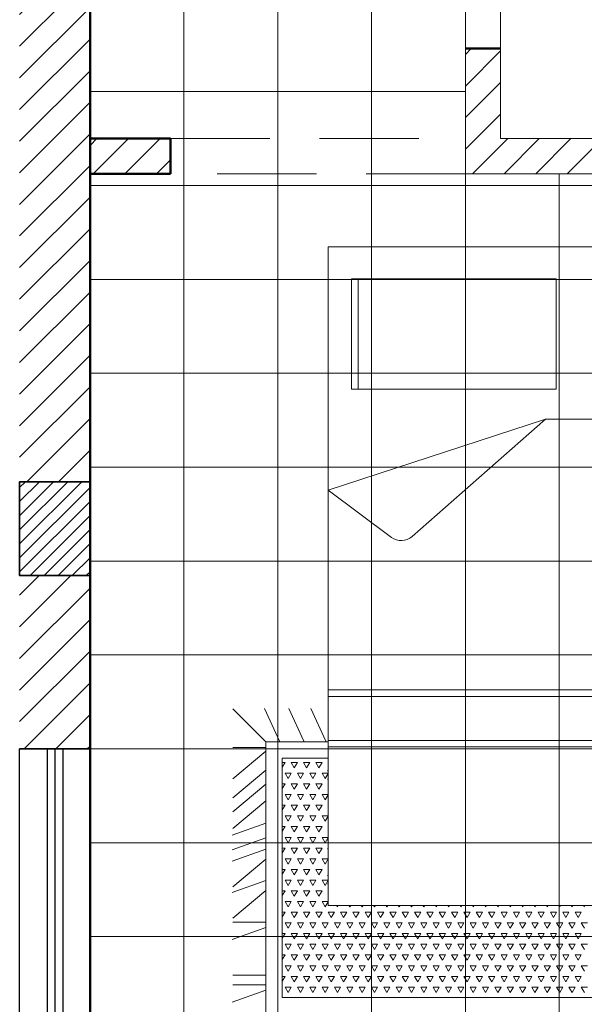
# Model space of a CAD drawing. Units: millimetres. Extents: x 225995 to 227247, y 225507 to 226008.
# Tile 14 of 23: x 226749 to 226821, y 225755 to 225881. Entities that reach past the tile are written whole.
import ezdxf

# ---------------------------------------------------------------- set-up
doc = ezdxf.new("R2010")
doc.units = ezdxf.units.MM
doc.linetypes.add('DASHED', pattern=[19.05, 12.7, -6.35])
for name, color, linetype, lineweight in [('A-COLS', 40, 'Continuous', 35), ('A-FLOR-PATT', 8, 'Continuous', 13), ('A-FURN', 9, 'Continuous', 18), ('A-GLAZ', 4, 'Continuous', 25), ('A-WALL', 7, 'Continuous', 50), ('A-WALL-OVHD', 1, 'DASHED', 18), ('A-WALL-PATT', 8, 'Continuous', 13)]:
    doc.layers.add(name, color=color, linetype=linetype, lineweight=lineweight)

# ---------------------------------------------------------------- blocks, each defined once
blk = doc.blocks.new('A$C6D2A2628')
for p, q in [((0.291, 2.4297), (1.791, 2.4297)), ((0.291, 0.4297), (0.291, 2.4297)), ((0.3622, 2.3321), (0.9834, 2.3321)), ((0.3622, 1.9967), (0.3622, 2.3321)), ((0.3822, 1.9967), (0.3822, 2.3321)), ((0.9834, 2.3321), (0.9834, 1.9967)), ((0.9834, 1.9967), (0.3622, 1.9967)), ((0.291, 1.6908), (0.9515, 1.9058)), ((0.9515, 1.9058), (0.5462, 1.5497)), ((0.9515, 1.9058), (1.1116, 1.9058)), ((0.4832, 1.5472), (0.291, 1.6908)), ((0.291, 1.0837), (1.791, 1.0837)), ((0.291, 1.0637), (1.791, 1.0637)), ((0.1019, 0.9267), (0.0019, 1.0267)), ((0.0977, 1.0278), (0.1431, 0.9278)), ((0.1716, 1.0278), (0.217, 0.9278)), ((0.2388, 1.0278), (0.2843, 0.9278)), ((0.291, 0.9307), (1.791, 0.9307)), ((0.0015, 0.9091), (0.1015, 0.9091)), ((0.0015, 0.8141), (0.1015, 0.8978)), ((0.291, 0.9267), (0.1019, 0.9267)), ((0.1019, 0.9267), (0.1019, 0.1)), ((0.291, 0.9107), (1.791, 0.9107)), ((0.291, 0.8767), (0.1519, 0.8767)), ((0.1519, 0.8767), (0.1519, 0.15)), ((0.0015, 0.7564), (0.1015, 0.84)), ((0.1519, 0.8494), (0.1601, 0.8636)), ((0.1519, 0.8636), (0.1601, 0.8636)), ((0.1882, 0.8473), (0.1788, 0.8636)), ((0.1788, 0.8636), (0.1976, 0.8636)), ((0.1882, 0.8473), (0.1976, 0.8636)), ((0.2257, 0.8473), (0.2163, 0.8636)), ((0.2163, 0.8636), (0.2351, 0.8636)), ((0.2257, 0.8473), (0.2351, 0.8636)), ((0.2632, 0.8473), (0.2538, 0.8636)), ((0.2538, 0.8636), (0.2726, 0.8636)), ((0.2632, 0.8473), (0.2726, 0.8636)), ((0.291, 0.8376), (0.2893, 0.8393)), ((0.1695, 0.8148), (0.1601, 0.8311)), ((0.1601, 0.8311), (0.1788, 0.8311)), ((0.1695, 0.8148), (0.1788, 0.8311)), ((0.207, 0.8148), (0.1976, 0.8311)), ((0.1976, 0.8311), (0.2163, 0.8311)), ((0.207, 0.8148), (0.2163, 0.8311)), ((0.2445, 0.8148), (0.2351, 0.8311)), ((0.2351, 0.8311), (0.2538, 0.8311)), ((0.2445, 0.8148), (0.2538, 0.8311)), ((0.282, 0.8148), (0.2726, 0.8311)), ((0.2726, 0.8311), (0.291, 0.8311)), ((0.282, 0.8148), (0.291, 0.8305)), ((0.291, 0.8144), (0.2893, 0.8128)), ((0.0015, 0.7139), (0.1015, 0.7975)), ((0.1519, 0.7844), (0.1601, 0.7986)), ((0.1519, 0.7986), (0.1601, 0.7986)), ((0.1882, 0.7824), (0.1788, 0.7986)), ((0.1788, 0.7986), (0.1976, 0.7986)), ((0.1882, 0.7824), (0.1976, 0.7986)), ((0.2257, 0.7824), (0.2163, 0.7986)), ((0.2163, 0.7986), (0.2351, 0.7986)), ((0.2257, 0.7824), (0.2351, 0.7986)), ((0.2632, 0.7824), (0.2538, 0.7986)), ((0.2538, 0.7986), (0.2726, 0.7986)), ((0.2632, 0.7824), (0.2726, 0.7986)), ((0.1695, 0.7499), (0.1601, 0.7661)), ((0.1601, 0.7661), (0.1788, 0.7661)), ((0.1695, 0.7499), (0.1788, 0.7661)), ((0.207, 0.7499), (0.1976, 0.7661)), ((0.1976, 0.7661), (0.2163, 0.7661)), ((0.207, 0.7499), (0.2163, 0.7661)), ((0.2445, 0.7499), (0.2351, 0.7661)), ((0.2351, 0.7661), (0.2538, 0.7661)), ((0.2445, 0.7499), (0.2538, 0.7661)), ((0.282, 0.7499), (0.2726, 0.7661)), ((0.2726, 0.7661), (0.291, 0.7661)), ((0.282, 0.7499), (0.291, 0.7655)), ((0.0015, 0.6633), (0.1015, 0.7469)), ((0.1519, 0.7195), (0.1601, 0.7337)), ((0.1519, 0.7337), (0.1601, 0.7337)), ((0.1882, 0.7174), (0.1788, 0.7337)), ((0.1788, 0.7337), (0.1976, 0.7337)), ((0.1882, 0.7174), (0.1976, 0.7337)), ((0.2257, 0.7174), (0.2163, 0.7337)), ((0.2163, 0.7337), (0.2351, 0.7337)), ((0.2257, 0.7174), (0.2351, 0.7337)), ((0.2632, 0.7174), (0.2538, 0.7337)), ((0.2538, 0.7337), (0.2726, 0.7337)), ((0.2632, 0.7174), (0.2726, 0.7337)), ((0.1695, 0.6849), (0.1601, 0.7012)), ((0.1601, 0.7012), (0.1788, 0.7012)), ((0.1695, 0.6849), (0.1788, 0.7012)), ((0.207, 0.6849), (0.1976, 0.7012)), ((0.1976, 0.7012), (0.2163, 0.7012)), ((0.207, 0.6849), (0.2163, 0.7012)), ((0.2445, 0.6849), (0.2351, 0.7012)), ((0.2351, 0.7012), (0.2538, 0.7012)), ((0.2445, 0.6849), (0.2538, 0.7012)), ((0.282, 0.6849), (0.2726, 0.7012)), ((0.2726, 0.7012), (0.291, 0.7012)), ((0.282, 0.6849), (0.291, 0.7006)), ((0, 0.6428), (0.1015, 0.6794)), ((0.1519, 0.6545), (0.1601, 0.6687)), ((0.1519, 0.6687), (0.1601, 0.6687)), ((0.1882, 0.6525), (0.1788, 0.6687)), ((0.1788, 0.6687), (0.1976, 0.6687)), ((0.1882, 0.6525), (0.1976, 0.6687)), ((0.2257, 0.6525), (0.2163, 0.6687)), ((0.2163, 0.6687), (0.2351, 0.6687)), ((0.2257, 0.6525), (0.2351, 0.6687)), ((0.2632, 0.6525), (0.2538, 0.6687)), ((0.2538, 0.6687), (0.2726, 0.6687)), ((0.2632, 0.6525), (0.2726, 0.6687)), ((0, 0.5984), (0.1015, 0.6351)), ((0.1695, 0.62), (0.1601, 0.6362)), ((0.1601, 0.6362), (0.1788, 0.6362)), ((0.1695, 0.62), (0.1788, 0.6362)), ((0.207, 0.62), (0.1976, 0.6362)), ((0.1976, 0.6362), (0.2163, 0.6362)), ((0.207, 0.62), (0.2163, 0.6362)), ((0.2445, 0.62), (0.2351, 0.6362)), ((0.2351, 0.6362), (0.2538, 0.6362)), ((0.2445, 0.62), (0.2538, 0.6362)), ((0.282, 0.62), (0.2726, 0.6362)), ((0.2726, 0.6362), (0.291, 0.6362)), ((0.282, 0.62), (0.291, 0.6356)), ((0, 0.5636), (0.1015, 0.6003)), ((0.1519, 0.5896), (0.1601, 0.6037)), ((0.1519, 0.6037), (0.1601, 0.6037)), ((0.1882, 0.5875), (0.1788, 0.6037)), ((0.1788, 0.6037), (0.1976, 0.6037)), ((0.1882, 0.5875), (0.1976, 0.6037)), ((0.2257, 0.5875), (0.2163, 0.6037)), ((0.2163, 0.6037), (0.2351, 0.6037)), ((0.2257, 0.5875), (0.2351, 0.6037)), ((0.2632, 0.5875), (0.2538, 0.6037)), ((0.2538, 0.6037), (0.2726, 0.6037)), ((0.2632, 0.5875), (0.2726, 0.6037)), ((0.291, 0.6255), (0.2893, 0.6271)), ((0.291, 0.6023), (0.2893, 0.6006)), ((0.0015, 0.4859), (0.1015, 0.5695)), ((0.1695, 0.555), (0.1601, 0.5713)), ((0.1601, 0.5713), (0.1788, 0.5713)), ((0.1695, 0.555), (0.1788, 0.5713)), ((0.207, 0.555), (0.1976, 0.5713)), ((0.1976, 0.5713), (0.2163, 0.5713)), ((0.207, 0.555), (0.2163, 0.5713)), ((0.2445, 0.555), (0.2351, 0.5713)), ((0.2351, 0.5713), (0.2538, 0.5713)), ((0.2445, 0.555), (0.2538, 0.5713)), ((0.282, 0.555), (0.2726, 0.5713)), ((0.2726, 0.5713), (0.291, 0.5713)), ((0.282, 0.555), (0.291, 0.5707)), ((0.1519, 0.5246), (0.1601, 0.5388)), ((0.1519, 0.5388), (0.1601, 0.5388)), ((0.1882, 0.5226), (0.1788, 0.5388)), ((0.1788, 0.5388), (0.1976, 0.5388)), ((0.1882, 0.5226), (0.1976, 0.5388)), ((0.2257, 0.5226), (0.2163, 0.5388)), ((0.2163, 0.5388), (0.2351, 0.5388)), ((0.2257, 0.5226), (0.2351, 0.5388)), ((0.2632, 0.5226), (0.2538, 0.5388)), ((0.2538, 0.5388), (0.2726, 0.5388)), ((0.2632, 0.5226), (0.2726, 0.5388)), ((0.291, 0.5194), (0.2893, 0.5211)), ((0, 0.4686), (0.1015, 0.5053)), ((0.1695, 0.4901), (0.1601, 0.5063)), ((0.1601, 0.5063), (0.1788, 0.5063)), ((0.1695, 0.4901), (0.1788, 0.5063)), ((0.207, 0.4901), (0.1976, 0.5063)), ((0.1976, 0.5063), (0.2163, 0.5063)), ((0.207, 0.4901), (0.2163, 0.5063)), ((0.2445, 0.4901), (0.2351, 0.5063)), ((0.2351, 0.5063), (0.2538, 0.5063)), ((0.2445, 0.4901), (0.2538, 0.5063)), ((0.282, 0.4901), (0.2726, 0.5063)), ((0.2726, 0.5063), (0.291, 0.5063)), ((0.282, 0.4901), (0.291, 0.5057)), ((0.291, 0.4962), (0.2893, 0.4946)), ((0.0015, 0.3909), (0.1015, 0.4745)), ((0.1519, 0.4597), (0.1601, 0.4738)), ((0.1519, 0.4738), (0.1601, 0.4738)), ((0.1882, 0.4576), (0.1788, 0.4738)), ((0.1788, 0.4738), (0.1976, 0.4738)), ((0.1882, 0.4576), (0.1976, 0.4738)), ((0.2257, 0.4576), (0.2163, 0.4738)), ((0.2163, 0.4738), (0.2351, 0.4738)), ((0.2257, 0.4576), (0.2351, 0.4738)), ((0.2632, 0.4576), (0.2538, 0.4738)), ((0.2538, 0.4738), (0.2726, 0.4738)), ((0.2632, 0.4576), (0.2726, 0.4738)), ((0.1695, 0.4251), (0.1601, 0.4414)), ((0.1601, 0.4414), (0.1788, 0.4414)), ((0.1695, 0.4251), (0.1788, 0.4414)), ((0.207, 0.4251), (0.1976, 0.4414)), ((0.1976, 0.4414), (0.2163, 0.4414)), ((0.207, 0.4251), (0.2163, 0.4414)), ((0.2445, 0.4251), (0.2351, 0.4414)), ((0.2351, 0.4414), (0.2538, 0.4414)), ((0.2445, 0.4251), (0.2538, 0.4414)), ((0.282, 0.4251), (0.2726, 0.4414)), ((0.2726, 0.4414), (0.291, 0.4414)), ((0.282, 0.4251), (0.291, 0.4408)), ((1.791, 0.4297), (0.291, 0.4297)), ((0.3195, 0.4251), (0.3168, 0.4297)), ((0.3195, 0.4251), (0.3221, 0.4297)), ((0.357, 0.4251), (0.3543, 0.4297)), ((0.357, 0.4251), (0.3596, 0.4297)), ((0.3945, 0.4251), (0.3918, 0.4297)), ((0.3945, 0.4251), (0.3971, 0.4297)), ((0.432, 0.4251), (0.4293, 0.4297)), ((0.432, 0.4251), (0.4346, 0.4297)), ((0.4695, 0.4251), (0.4668, 0.4297)), ((0.4695, 0.4251), (0.4721, 0.4297)), ((0.507, 0.4251), (0.5043, 0.4297)), ((0.507, 0.4251), (0.5096, 0.4297)), ((0.5445, 0.4251), (0.5418, 0.4297)), ((0.5445, 0.4251), (0.5471, 0.4297)), ((0.582, 0.4251), (0.5793, 0.4297)), ((0.582, 0.4251), (0.5846, 0.4297)), ((0.6195, 0.4251), (0.6168, 0.4297)), ((0.6195, 0.4251), (0.6221, 0.4297)), ((0.657, 0.4251), (0.6543, 0.4297)), ((0.657, 0.4251), (0.6596, 0.4297)), ((0.6945, 0.4251), (0.6918, 0.4297)), ((0.6945, 0.4251), (0.6971, 0.4297)), ((0.732, 0.4251), (0.7293, 0.4297)), ((0.732, 0.4251), (0.7346, 0.4297)), ((0.7695, 0.4251), (0.7668, 0.4297)), ((0.7695, 0.4251), (0.7721, 0.4297)), ((0.807, 0.4251), (0.8043, 0.4297)), ((0.807, 0.4251), (0.8096, 0.4297)), ((0.8445, 0.4251), (0.8418, 0.4297)), ((0.8445, 0.4251), (0.8471, 0.4297)), ((0.882, 0.4251), (0.8793, 0.4297)), ((0.882, 0.4251), (0.8846, 0.4297)), ((0.9195, 0.4251), (0.9168, 0.4297)), ((0.9195, 0.4251), (0.9221, 0.4297)), ((0.957, 0.4251), (0.9543, 0.4297)), ((0.957, 0.4251), (0.9596, 0.4297)), ((0.9945, 0.4251), (0.9918, 0.4297)), ((0.9945, 0.4251), (0.9971, 0.4297)), ((1.032, 0.4251), (1.0293, 0.4297)), ((1.032, 0.4251), (1.0346, 0.4297)), ((1.0695, 0.4251), (1.0668, 0.4297)), ((0.1519, 0.3947), (0.1601, 0.4089)), ((0.1519, 0.4089), (0.1601, 0.4089)), ((0.1882, 0.3927), (0.1788, 0.4089)), ((0.1788, 0.4089), (0.1976, 0.4089)), ((0.1882, 0.3927), (0.1976, 0.4089)), ((0.2257, 0.3927), (0.2163, 0.4089)), ((0.2163, 0.4089), (0.2351, 0.4089)), ((0.2257, 0.3927), (0.2351, 0.4089)), ((0.2632, 0.3927), (0.2538, 0.4089)), ((0.2538, 0.4089), (0.2726, 0.4089)), ((0.2632, 0.3927), (0.2726, 0.4089)), ((0.3007, 0.3927), (0.2913, 0.4089)), ((0.2913, 0.4089), (0.3101, 0.4089)), ((0.3007, 0.3927), (0.3101, 0.4089)), ((0.3382, 0.3927), (0.3288, 0.4089)), ((0.3288, 0.4089), (0.3476, 0.4089)), ((0.3382, 0.3927), (0.3476, 0.4089)), ((0.3757, 0.3927), (0.3663, 0.4089)), ((0.3663, 0.4089), (0.3851, 0.4089)), ((0.3757, 0.3927), (0.3851, 0.4089)), ((0.4132, 0.3927), (0.4038, 0.4089)), ((0.4038, 0.4089), (0.4226, 0.4089)), ((0.4132, 0.3927), (0.4226, 0.4089)), ((0.4507, 0.3927), (0.4413, 0.4089)), ((0.4413, 0.4089), (0.4601, 0.4089)), ((0.4507, 0.3927), (0.4601, 0.4089)), ((0.4882, 0.3927), (0.4788, 0.4089)), ((0.4788, 0.4089), (0.4976, 0.4089)), ((0.4882, 0.3927), (0.4976, 0.4089)), ((0.5257, 0.3927), (0.5163, 0.4089)), ((0.5163, 0.4089), (0.5351, 0.4089)), ((0.5257, 0.3927), (0.5351, 0.4089)), ((0.5632, 0.3927), (0.5538, 0.4089)), ((0.5538, 0.4089), (0.5726, 0.4089)), ((0.5632, 0.3927), (0.5726, 0.4089)), ((0.6007, 0.3927), (0.5913, 0.4089)), ((0.5913, 0.4089), (0.6101, 0.4089)), ((0.6007, 0.3927), (0.6101, 0.4089)), ((0.6382, 0.3927), (0.6288, 0.4089)), ((0.6288, 0.4089), (0.6476, 0.4089)), ((0.6382, 0.3927), (0.6476, 0.4089)), ((0.6757, 0.3927), (0.6663, 0.4089)), ((0.6663, 0.4089), (0.6851, 0.4089)), ((0.6757, 0.3927), (0.6851, 0.4089)), ((0.7132, 0.3927), (0.7038, 0.4089)), ((0.7038, 0.4089), (0.7226, 0.4089)), ((0.7132, 0.3927), (0.7226, 0.4089)), ((0.7507, 0.3927), (0.7413, 0.4089)), ((0.7413, 0.4089), (0.7601, 0.4089)), ((0.7507, 0.3927), (0.7601, 0.4089)), ((0.7882, 0.3927), (0.7788, 0.4089)), ((0.7788, 0.4089), (0.7976, 0.4089)), ((0.7882, 0.3927), (0.7976, 0.4089)), ((0.8257, 0.3927), (0.8163, 0.4089)), ((0.8163, 0.4089), (0.8351, 0.4089)), ((0.8257, 0.3927), (0.8351, 0.4089)), ((0.8632, 0.3927), (0.8538, 0.4089)), ((0.8538, 0.4089), (0.8726, 0.4089)), ((0.8632, 0.3927), (0.8726, 0.4089)), ((0.9007, 0.3927), (0.8913, 0.4089)), ((0.8913, 0.4089), (0.9101, 0.4089)), ((0.9007, 0.3927), (0.9101, 0.4089)), ((0.9382, 0.3927), (0.9288, 0.4089)), ((0.9288, 0.4089), (0.9476, 0.4089)), ((0.9382, 0.3927), (0.9476, 0.4089)), ((0.9757, 0.3927), (0.9663, 0.4089)), ((0.9663, 0.4089), (0.9851, 0.4089)), ((0.9757, 0.3927), (0.9851, 0.4089)), ((1.0132, 0.3927), (1.0038, 0.4089)), ((1.0038, 0.4089), (1.0226, 0.4089)), ((1.0132, 0.3927), (1.0226, 0.4089)), ((1.0507, 0.3927), (1.0413, 0.4089)), ((1.0413, 0.4089), (1.0601, 0.4089)), ((1.0507, 0.3927), (1.0601, 0.4089)), ((0, 0.3261), (0.1015, 0.3628)), ((0.0015, 0.3783), (0.1015, 0.3783)), ((0.1695, 0.3602), (0.1601, 0.3764)), ((0.1601, 0.3764), (0.1788, 0.3764)), ((0.1695, 0.3602), (0.1788, 0.3764)), ((0.207, 0.3602), (0.1976, 0.3764)), ((0.1976, 0.3764), (0.2163, 0.3764)), ((0.207, 0.3602), (0.2163, 0.3764)), ((0.2445, 0.3602), (0.2351, 0.3764)), ((0.2351, 0.3764), (0.2538, 0.3764)), ((0.2445, 0.3602), (0.2538, 0.3764)), ((0.282, 0.3602), (0.2726, 0.3764)), ((0.2726, 0.3764), (0.2913, 0.3764)), ((0.282, 0.3602), (0.2913, 0.3764)), ((0.3195, 0.3602), (0.3101, 0.3764)), ((0.3101, 0.3764), (0.3288, 0.3764)), ((0.3195, 0.3602), (0.3288, 0.3764)), ((0.357, 0.3602), (0.3476, 0.3764)), ((0.3476, 0.3764), (0.3663, 0.3764)), ((0.357, 0.3602), (0.3663, 0.3764)), ((0.3945, 0.3602), (0.3851, 0.3764)), ((0.3851, 0.3764), (0.4038, 0.3764)), ((0.3945, 0.3602), (0.4038, 0.3764)), ((0.432, 0.3602), (0.4226, 0.3764)), ((0.4226, 0.3764), (0.4413, 0.3764)), ((0.432, 0.3602), (0.4413, 0.3764)), ((0.4695, 0.3602), (0.4601, 0.3764)), ((0.4601, 0.3764), (0.4788, 0.3764)), ((0.4695, 0.3602), (0.4788, 0.3764)), ((0.507, 0.3602), (0.4976, 0.3764)), ((0.4976, 0.3764), (0.5163, 0.3764)), ((0.507, 0.3602), (0.5163, 0.3764)), ((0.5445, 0.3602), (0.5351, 0.3764)), ((0.5351, 0.3764), (0.5538, 0.3764)), ((0.5445, 0.3602), (0.5538, 0.3764)), ((0.582, 0.3602), (0.5726, 0.3764)), ((0.5726, 0.3764), (0.5913, 0.3764)), ((0.582, 0.3602), (0.5913, 0.3764)), ((0.6195, 0.3602), (0.6101, 0.3764)), ((0.6101, 0.3764), (0.6288, 0.3764)), ((0.6195, 0.3602), (0.6288, 0.3764)), ((0.657, 0.3602), (0.6476, 0.3764)), ((0.6476, 0.3764), (0.6663, 0.3764)), ((0.657, 0.3602), (0.6663, 0.3764)), ((0.6945, 0.3602), (0.6851, 0.3764)), ((0.6851, 0.3764), (0.7038, 0.3764)), ((0.6945, 0.3602), (0.7038, 0.3764)), ((0.732, 0.3602), (0.7226, 0.3764)), ((0.7226, 0.3764), (0.7413, 0.3764)), ((0.732, 0.3602), (0.7413, 0.3764)), ((0.7695, 0.3602), (0.7601, 0.3764)), ((0.7601, 0.3764), (0.7788, 0.3764)), ((0.7695, 0.3602), (0.7788, 0.3764)), ((0.807, 0.3602), (0.7976, 0.3764)), ((0.7976, 0.3764), (0.8163, 0.3764)), ((0.807, 0.3602), (0.8163, 0.3764)), ((0.8445, 0.3602), (0.8351, 0.3764)), ((0.8351, 0.3764), (0.8538, 0.3764)), ((0.8445, 0.3602), (0.8538, 0.3764)), ((0.882, 0.3602), (0.8726, 0.3764)), ((0.8726, 0.3764), (0.8913, 0.3764)), ((0.882, 0.3602), (0.8913, 0.3764)), ((0.9195, 0.3602), (0.9101, 0.3764)), ((0.9101, 0.3764), (0.9288, 0.3764)), ((0.9195, 0.3602), (0.9288, 0.3764)), ((0.957, 0.3602), (0.9476, 0.3764)), ((0.9476, 0.3764), (0.9663, 0.3764)), ((0.957, 0.3602), (0.9663, 0.3764)), ((0.9945, 0.3602), (0.9851, 0.3764)), ((0.9851, 0.3764), (1.0038, 0.3764)), ((0.9945, 0.3602), (1.0038, 0.3764)), ((1.032, 0.3602), (1.0226, 0.3764)), ((1.0226, 0.3764), (1.0413, 0.3764)), ((1.032, 0.3602), (1.0413, 0.3764)), ((1.0695, 0.3602), (1.0601, 0.3764)), ((1.0601, 0.3764), (1.0788, 0.3764)), ((0.1519, 0.3298), (0.1601, 0.3439)), ((0.1519, 0.3439), (0.1601, 0.3439)), ((0.1882, 0.3277), (0.1788, 0.3439)), ((0.1788, 0.3439), (0.1976, 0.3439)), ((0.1882, 0.3277), (0.1976, 0.3439)), ((0.2257, 0.3277), (0.2163, 0.3439)), ((0.2163, 0.3439), (0.2351, 0.3439)), ((0.2257, 0.3277), (0.2351, 0.3439)), ((0.2632, 0.3277), (0.2538, 0.3439)), ((0.2538, 0.3439), (0.2726, 0.3439)), ((0.2632, 0.3277), (0.2726, 0.3439)), ((0.3007, 0.3277), (0.2913, 0.3439)), ((0.2913, 0.3439), (0.3101, 0.3439)), ((0.3007, 0.3277), (0.3101, 0.3439)), ((0.3382, 0.3277), (0.3288, 0.3439)), ((0.3288, 0.3439), (0.3476, 0.3439)), ((0.3382, 0.3277), (0.3476, 0.3439)), ((0.3757, 0.3277), (0.3663, 0.3439)), ((0.3663, 0.3439), (0.3851, 0.3439)), ((0.3757, 0.3277), (0.3851, 0.3439)), ((0.4132, 0.3277), (0.4038, 0.3439)), ((0.4038, 0.3439), (0.4226, 0.3439)), ((0.4132, 0.3277), (0.4226, 0.3439)), ((0.4507, 0.3277), (0.4413, 0.3439)), ((0.4413, 0.3439), (0.4601, 0.3439)), ((0.4507, 0.3277), (0.4601, 0.3439)), ((0.4882, 0.3277), (0.4788, 0.3439)), ((0.4788, 0.3439), (0.4976, 0.3439)), ((0.4882, 0.3277), (0.4976, 0.3439)), ((0.5257, 0.3277), (0.5163, 0.3439)), ((0.5163, 0.3439), (0.5351, 0.3439)), ((0.5257, 0.3277), (0.5351, 0.3439)), ((0.5632, 0.3277), (0.5538, 0.3439)), ((0.5538, 0.3439), (0.5726, 0.3439)), ((0.5632, 0.3277), (0.5726, 0.3439)), ((0.6007, 0.3277), (0.5913, 0.3439)), ((0.5913, 0.3439), (0.6101, 0.3439)), ((0.6007, 0.3277), (0.6101, 0.3439)), ((0.6382, 0.3277), (0.6288, 0.3439)), ((0.6288, 0.3439), (0.6476, 0.3439)), ((0.6382, 0.3277), (0.6476, 0.3439)), ((0.6757, 0.3277), (0.6663, 0.3439)), ((0.6663, 0.3439), (0.6851, 0.3439)), ((0.6757, 0.3277), (0.6851, 0.3439)), ((0.7132, 0.3277), (0.7038, 0.3439)), ((0.7038, 0.3439), (0.7226, 0.3439)), ((0.7132, 0.3277), (0.7226, 0.3439)), ((0.7507, 0.3277), (0.7413, 0.3439)), ((0.7413, 0.3439), (0.7601, 0.3439)), ((0.7507, 0.3277), (0.7601, 0.3439)), ((0.7882, 0.3277), (0.7788, 0.3439)), ((0.7788, 0.3439), (0.7976, 0.3439)), ((0.7882, 0.3277), (0.7976, 0.3439)), ((0.8257, 0.3277), (0.8163, 0.3439)), ((0.8163, 0.3439), (0.8351, 0.3439)), ((0.8257, 0.3277), (0.8351, 0.3439)), ((0.8632, 0.3277), (0.8538, 0.3439)), ((0.8538, 0.3439), (0.8726, 0.3439)), ((0.8632, 0.3277), (0.8726, 0.3439)), ((0.9007, 0.3277), (0.8913, 0.3439)), ((0.8913, 0.3439), (0.9101, 0.3439)), ((0.9007, 0.3277), (0.9101, 0.3439)), ((0.9382, 0.3277), (0.9288, 0.3439)), ((0.9288, 0.3439), (0.9476, 0.3439)), ((0.9382, 0.3277), (0.9476, 0.3439)), ((0.9757, 0.3277), (0.9663, 0.3439)), ((0.9663, 0.3439), (0.9851, 0.3439)), ((0.9757, 0.3277), (0.9851, 0.3439)), ((1.0132, 0.3277), (1.0038, 0.3439)), ((1.0038, 0.3439), (1.0226, 0.3439)), ((1.0132, 0.3277), (1.0226, 0.3439)), ((1.0507, 0.3277), (1.0413, 0.3439)), ((1.0413, 0.3439), (1.0601, 0.3439)), ((1.0507, 0.3277), (1.0601, 0.3439)), ((0.1695, 0.2952), (0.1601, 0.3115)), ((0.1601, 0.3115), (0.1788, 0.3115)), ((0.1695, 0.2952), (0.1788, 0.3115)), ((0.207, 0.2952), (0.1976, 0.3115)), ((0.1976, 0.3115), (0.2163, 0.3115)), ((0.207, 0.2952), (0.2163, 0.3115)), ((0.2445, 0.2952), (0.2351, 0.3115)), ((0.2351, 0.3115), (0.2538, 0.3115)), ((0.2445, 0.2952), (0.2538, 0.3115)), ((0.282, 0.2952), (0.2726, 0.3115)), ((0.2726, 0.3115), (0.2913, 0.3115)), ((0.282, 0.2952), (0.2913, 0.3115)), ((0.3195, 0.2952), (0.3101, 0.3115)), ((0.3101, 0.3115), (0.3288, 0.3115)), ((0.3195, 0.2952), (0.3288, 0.3115)), ((0.357, 0.2952), (0.3476, 0.3115)), ((0.3476, 0.3115), (0.3663, 0.3115)), ((0.357, 0.2952), (0.3663, 0.3115)), ((0.3945, 0.2952), (0.3851, 0.3115)), ((0.3851, 0.3115), (0.4038, 0.3115)), ((0.3945, 0.2952), (0.4038, 0.3115)), ((0.432, 0.2952), (0.4226, 0.3115)), ((0.4226, 0.3115), (0.4413, 0.3115)), ((0.432, 0.2952), (0.4413, 0.3115)), ((0.4695, 0.2952), (0.4601, 0.3115)), ((0.4601, 0.3115), (0.4788, 0.3115)), ((0.4695, 0.2952), (0.4788, 0.3115)), ((0.507, 0.2952), (0.4976, 0.3115)), ((0.4976, 0.3115), (0.5163, 0.3115)), ((0.507, 0.2952), (0.5163, 0.3115)), ((0.5445, 0.2952), (0.5351, 0.3115)), ((0.5351, 0.3115), (0.5538, 0.3115)), ((0.5445, 0.2952), (0.5538, 0.3115)), ((0.582, 0.2952), (0.5726, 0.3115)), ((0.5726, 0.3115), (0.5913, 0.3115)), ((0.582, 0.2952), (0.5913, 0.3115)), ((0.6195, 0.2952), (0.6101, 0.3115)), ((0.6101, 0.3115), (0.6288, 0.3115)), ((0.6195, 0.2952), (0.6288, 0.3115)), ((0.657, 0.2952), (0.6476, 0.3115)), ((0.6476, 0.3115), (0.6663, 0.3115)), ((0.657, 0.2952), (0.6663, 0.3115)), ((0.6945, 0.2952), (0.6851, 0.3115)), ((0.6851, 0.3115), (0.7038, 0.3115)), ((0.6945, 0.2952), (0.7038, 0.3115)), ((0.732, 0.2952), (0.7226, 0.3115)), ((0.7226, 0.3115), (0.7413, 0.3115)), ((0.732, 0.2952), (0.7413, 0.3115)), ((0.7695, 0.2952), (0.7601, 0.3115)), ((0.7601, 0.3115), (0.7788, 0.3115)), ((0.7695, 0.2952), (0.7788, 0.3115)), ((0.807, 0.2952), (0.7976, 0.3115)), ((0.7976, 0.3115), (0.8163, 0.3115)), ((0.807, 0.2952), (0.8163, 0.3115)), ((0.8445, 0.2952), (0.8351, 0.3115)), ((0.8351, 0.3115), (0.8538, 0.3115)), ((0.8445, 0.2952), (0.8538, 0.3115)), ((0.882, 0.2952), (0.8726, 0.3115)), ((0.8726, 0.3115), (0.8913, 0.3115)), ((0.882, 0.2952), (0.8913, 0.3115)), ((0.9195, 0.2952), (0.9101, 0.3115)), ((0.9101, 0.3115), (0.9288, 0.3115)), ((0.9195, 0.2952), (0.9288, 0.3115)), ((0.957, 0.2952), (0.9476, 0.3115)), ((0.9476, 0.3115), (0.9663, 0.3115)), ((0.957, 0.2952), (0.9663, 0.3115)), ((0.9945, 0.2952), (0.9851, 0.3115)), ((0.9851, 0.3115), (1.0038, 0.3115)), ((0.9945, 0.2952), (1.0038, 0.3115)), ((1.032, 0.2952), (1.0226, 0.3115)), ((1.0226, 0.3115), (1.0413, 0.3115)), ((1.032, 0.2952), (1.0413, 0.3115)), ((1.0695, 0.2952), (1.0601, 0.3115)), ((1.0601, 0.3115), (1.0788, 0.3115)), ((0.1519, 0.2648), (0.1601, 0.279)), ((0.1519, 0.279), (0.1601, 0.279)), ((0.1882, 0.2628), (0.1788, 0.279)), ((0.1788, 0.279), (0.1976, 0.279)), ((0.1882, 0.2628), (0.1976, 0.279)), ((0.2257, 0.2628), (0.2163, 0.279)), ((0.2163, 0.279), (0.2351, 0.279)), ((0.2257, 0.2628), (0.2351, 0.279)), ((0.2632, 0.2628), (0.2538, 0.279)), ((0.2538, 0.279), (0.2726, 0.279)), ((0.2632, 0.2628), (0.2726, 0.279)), ((0.3007, 0.2628), (0.2913, 0.279)), ((0.2913, 0.279), (0.3101, 0.279)), ((0.3007, 0.2628), (0.3101, 0.279)), ((0.3382, 0.2628), (0.3288, 0.279)), ((0.3288, 0.279), (0.3476, 0.279)), ((0.3382, 0.2628), (0.3476, 0.279)), ((0.3757, 0.2628), (0.3663, 0.279)), ((0.3663, 0.279), (0.3851, 0.279)), ((0.3757, 0.2628), (0.3851, 0.279)), ((0.4132, 0.2628), (0.4038, 0.279)), ((0.4038, 0.279), (0.4226, 0.279)), ((0.4132, 0.2628), (0.4226, 0.279)), ((0.4507, 0.2628), (0.4413, 0.279)), ((0.4413, 0.279), (0.4601, 0.279)), ((0.4507, 0.2628), (0.4601, 0.279)), ((0.4882, 0.2628), (0.4788, 0.279)), ((0.4788, 0.279), (0.4976, 0.279)), ((0.4882, 0.2628), (0.4976, 0.279)), ((0.5257, 0.2628), (0.5163, 0.279)), ((0.5163, 0.279), (0.5351, 0.279)), ((0.5257, 0.2628), (0.5351, 0.279)), ((0.5632, 0.2628), (0.5538, 0.279)), ((0.5538, 0.279), (0.5726, 0.279)), ((0.5632, 0.2628), (0.5726, 0.279)), ((0.6007, 0.2628), (0.5913, 0.279)), ((0.5913, 0.279), (0.6101, 0.279)), ((0.6007, 0.2628), (0.6101, 0.279)), ((0.6382, 0.2628), (0.6288, 0.279)), ((0.6288, 0.279), (0.6476, 0.279)), ((0.6382, 0.2628), (0.6476, 0.279)), ((0.6757, 0.2628), (0.6663, 0.279)), ((0.6663, 0.279), (0.6851, 0.279)), ((0.6757, 0.2628), (0.6851, 0.279)), ((0.7132, 0.2628), (0.7038, 0.279)), ((0.7038, 0.279), (0.7226, 0.279)), ((0.7132, 0.2628), (0.7226, 0.279)), ((0.7507, 0.2628), (0.7413, 0.279)), ((0.7413, 0.279), (0.7601, 0.279)), ((0.7507, 0.2628), (0.7601, 0.279)), ((0.7882, 0.2628), (0.7788, 0.279)), ((0.7788, 0.279), (0.7976, 0.279)), ((0.7882, 0.2628), (0.7976, 0.279)), ((0.8257, 0.2628), (0.8163, 0.279)), ((0.8163, 0.279), (0.8351, 0.279)), ((0.8257, 0.2628), (0.8351, 0.279)), ((0.8632, 0.2628), (0.8538, 0.279)), ((0.8538, 0.279), (0.8726, 0.279)), ((0.8632, 0.2628), (0.8726, 0.279)), ((0.9007, 0.2628), (0.8913, 0.279)), ((0.8913, 0.279), (0.9101, 0.279)), ((0.9007, 0.2628), (0.9101, 0.279)), ((0.9382, 0.2628), (0.9288, 0.279)), ((0.9288, 0.279), (0.9476, 0.279)), ((0.9382, 0.2628), (0.9476, 0.279)), ((0.9757, 0.2628), (0.9663, 0.279)), ((0.9663, 0.279), (0.9851, 0.279)), ((0.9757, 0.2628), (0.9851, 0.279)), ((1.0132, 0.2628), (1.0038, 0.279)), ((1.0038, 0.279), (1.0226, 0.279)), ((1.0132, 0.2628), (1.0226, 0.279)), ((1.0507, 0.2628), (1.0413, 0.279)), ((1.0413, 0.279), (1.0601, 0.279)), ((1.0507, 0.2628), (1.0601, 0.279)), ((0.1695, 0.2303), (0.1601, 0.2465)), ((0.1601, 0.2465), (0.1788, 0.2465)), ((0.1695, 0.2303), (0.1788, 0.2465)), ((0.207, 0.2303), (0.1976, 0.2465)), ((0.1976, 0.2465), (0.2163, 0.2465)), ((0.207, 0.2303), (0.2163, 0.2465)), ((0.2445, 0.2303), (0.2351, 0.2465)), ((0.2351, 0.2465), (0.2538, 0.2465)), ((0.2445, 0.2303), (0.2538, 0.2465)), ((0.282, 0.2303), (0.2726, 0.2465)), ((0.2726, 0.2465), (0.2913, 0.2465)), ((0.282, 0.2303), (0.2913, 0.2465)), ((0.3195, 0.2303), (0.3101, 0.2465)), ((0.3101, 0.2465), (0.3288, 0.2465)), ((0.3195, 0.2303), (0.3288, 0.2465)), ((0.357, 0.2303), (0.3476, 0.2465)), ((0.3476, 0.2465), (0.3663, 0.2465)), ((0.357, 0.2303), (0.3663, 0.2465)), ((0.3945, 0.2303), (0.3851, 0.2465)), ((0.3851, 0.2465), (0.4038, 0.2465)), ((0.3945, 0.2303), (0.4038, 0.2465)), ((0.432, 0.2303), (0.4226, 0.2465)), ((0.4226, 0.2465), (0.4413, 0.2465)), ((0.432, 0.2303), (0.4413, 0.2465)), ((0.4695, 0.2303), (0.4601, 0.2465)), ((0.4601, 0.2465), (0.4788, 0.2465)), ((0.4695, 0.2303), (0.4788, 0.2465)), ((0.507, 0.2303), (0.4976, 0.2465)), ((0.4976, 0.2465), (0.5163, 0.2465)), ((0.507, 0.2303), (0.5163, 0.2465)), ((0.5445, 0.2303), (0.5351, 0.2465)), ((0.5351, 0.2465), (0.5538, 0.2465)), ((0.5445, 0.2303), (0.5538, 0.2465)), ((0.582, 0.2303), (0.5726, 0.2465)), ((0.5726, 0.2465), (0.5913, 0.2465)), ((0.582, 0.2303), (0.5913, 0.2465)), ((0.6195, 0.2303), (0.6101, 0.2465)), ((0.6101, 0.2465), (0.6288, 0.2465)), ((0.6195, 0.2303), (0.6288, 0.2465)), ((0.657, 0.2303), (0.6476, 0.2465)), ((0.6476, 0.2465), (0.6663, 0.2465)), ((0.657, 0.2303), (0.6663, 0.2465)), ((0.6945, 0.2303), (0.6851, 0.2465)), ((0.6851, 0.2465), (0.7038, 0.2465)), ((0.6945, 0.2303), (0.7038, 0.2465)), ((0.732, 0.2303), (0.7226, 0.2465)), ((0.7226, 0.2465), (0.7413, 0.2465)), ((0.732, 0.2303), (0.7413, 0.2465)), ((0.7695, 0.2303), (0.7601, 0.2465)), ((0.7601, 0.2465), (0.7788, 0.2465)), ((0.7695, 0.2303), (0.7788, 0.2465)), ((0.807, 0.2303), (0.7976, 0.2465)), ((0.7976, 0.2465), (0.8163, 0.2465)), ((0.807, 0.2303), (0.8163, 0.2465)), ((0.8445, 0.2303), (0.8351, 0.2465)), ((0.8351, 0.2465), (0.8538, 0.2465)), ((0.8445, 0.2303), (0.8538, 0.2465)), ((0.882, 0.2303), (0.8726, 0.2465)), ((0.8726, 0.2465), (0.8913, 0.2465)), ((0.882, 0.2303), (0.8913, 0.2465)), ((0.9195, 0.2303), (0.9101, 0.2465)), ((0.9101, 0.2465), (0.9288, 0.2465)), ((0.9195, 0.2303), (0.9288, 0.2465)), ((0.957, 0.2303), (0.9476, 0.2465)), ((0.9476, 0.2465), (0.9663, 0.2465)), ((0.957, 0.2303), (0.9663, 0.2465)), ((0.9945, 0.2303), (0.9851, 0.2465)), ((0.9851, 0.2465), (1.0038, 0.2465)), ((0.9945, 0.2303), (1.0038, 0.2465)), ((1.032, 0.2303), (1.0226, 0.2465)), ((1.0226, 0.2465), (1.0413, 0.2465)), ((1.032, 0.2303), (1.0413, 0.2465)), ((1.0695, 0.2303), (1.0601, 0.2465)), ((1.0601, 0.2465), (1.0788, 0.2465)), ((0.0015, 0.2173), (0.1015, 0.2173)), ((0.1519, 0.1999), (0.1601, 0.214)), ((0.1519, 0.214), (0.1601, 0.214)), ((0.1882, 0.1978), (0.1788, 0.214)), ((0.1788, 0.214), (0.1976, 0.214)), ((0.1882, 0.1978), (0.1976, 0.214)), ((0.2257, 0.1978), (0.2163, 0.214)), ((0.2163, 0.214), (0.2351, 0.214)), ((0.2257, 0.1978), (0.2351, 0.214)), ((0.2632, 0.1978), (0.2538, 0.214)), ((0.2538, 0.214), (0.2726, 0.214)), ((0.2632, 0.1978), (0.2726, 0.214)), ((0.3007, 0.1978), (0.2913, 0.214)), ((0.2913, 0.214), (0.3101, 0.214)), ((0.3007, 0.1978), (0.3101, 0.214)), ((0.3382, 0.1978), (0.3288, 0.214)), ((0.3288, 0.214), (0.3476, 0.214)), ((0.3382, 0.1978), (0.3476, 0.214)), ((0.3757, 0.1978), (0.3663, 0.214)), ((0.3663, 0.214), (0.3851, 0.214)), ((0.3757, 0.1978), (0.3851, 0.214)), ((0.4132, 0.1978), (0.4038, 0.214)), ((0.4038, 0.214), (0.4226, 0.214)), ((0.4132, 0.1978), (0.4226, 0.214)), ((0.4507, 0.1978), (0.4413, 0.214)), ((0.4413, 0.214), (0.4601, 0.214)), ((0.4507, 0.1978), (0.4601, 0.214)), ((0.4882, 0.1978), (0.4788, 0.214)), ((0.4788, 0.214), (0.4976, 0.214)), ((0.4882, 0.1978), (0.4976, 0.214)), ((0.5257, 0.1978), (0.5163, 0.214)), ((0.5163, 0.214), (0.5351, 0.214)), ((0.5257, 0.1978), (0.5351, 0.214)), ((0.5632, 0.1978), (0.5538, 0.214)), ((0.5538, 0.214), (0.5726, 0.214)), ((0.5632, 0.1978), (0.5726, 0.214)), ((0.6007, 0.1978), (0.5913, 0.214)), ((0.5913, 0.214), (0.6101, 0.214)), ((0.6007, 0.1978), (0.6101, 0.214)), ((0.6382, 0.1978), (0.6288, 0.214)), ((0.6288, 0.214), (0.6476, 0.214)), ((0.6382, 0.1978), (0.6476, 0.214)), ((0.6757, 0.1978), (0.6663, 0.214)), ((0.6663, 0.214), (0.6851, 0.214)), ((0.6757, 0.1978), (0.6851, 0.214)), ((0.7132, 0.1978), (0.7038, 0.214)), ((0.7038, 0.214), (0.7226, 0.214)), ((0.7132, 0.1978), (0.7226, 0.214)), ((0.7507, 0.1978), (0.7413, 0.214)), ((0.7413, 0.214), (0.7601, 0.214)), ((0.7507, 0.1978), (0.7601, 0.214)), ((0.7882, 0.1978), (0.7788, 0.214)), ((0.7788, 0.214), (0.7976, 0.214)), ((0.7882, 0.1978), (0.7976, 0.214)), ((0.8257, 0.1978), (0.8163, 0.214)), ((0.8163, 0.214), (0.8351, 0.214)), ((0.8257, 0.1978), (0.8351, 0.214)), ((0.8632, 0.1978), (0.8538, 0.214)), ((0.8538, 0.214), (0.8726, 0.214)), ((0.8632, 0.1978), (0.8726, 0.214)), ((0.9007, 0.1978), (0.8913, 0.214)), ((0.8913, 0.214), (0.9101, 0.214)), ((0.9007, 0.1978), (0.9101, 0.214)), ((0.9382, 0.1978), (0.9288, 0.214)), ((0.9288, 0.214), (0.9476, 0.214)), ((0.9382, 0.1978), (0.9476, 0.214)), ((0.9757, 0.1978), (0.9663, 0.214)), ((0.9663, 0.214), (0.9851, 0.214)), ((0.9757, 0.1978), (0.9851, 0.214)), ((1.0132, 0.1978), (1.0038, 0.214)), ((1.0038, 0.214), (1.0226, 0.214)), ((1.0132, 0.1978), (1.0226, 0.214)), ((1.0507, 0.1978), (1.0413, 0.214)), ((1.0413, 0.214), (1.0601, 0.214)), ((1.0507, 0.1978), (1.0601, 0.214)), ((0.0015, 0.1884), (0.1015, 0.1884)), ((0.1695, 0.1653), (0.1601, 0.1816)), ((0.1601, 0.1816), (0.1788, 0.1816)), ((0.1695, 0.1653), (0.1788, 0.1816)), ((0.207, 0.1653), (0.1976, 0.1816)), ((0.1976, 0.1816), (0.2163, 0.1816)), ((0.207, 0.1653), (0.2163, 0.1816)), ((0.2445, 0.1653), (0.2351, 0.1816)), ((0.2351, 0.1816), (0.2538, 0.1816)), ((0.2445, 0.1653), (0.2538, 0.1816)), ((0.282, 0.1653), (0.2726, 0.1816)), ((0.2726, 0.1816), (0.2913, 0.1816)), ((0.282, 0.1653), (0.2913, 0.1816)), ((0.3195, 0.1653), (0.3101, 0.1816)), ((0.3101, 0.1816), (0.3288, 0.1816)), ((0.3195, 0.1653), (0.3288, 0.1816)), ((0.357, 0.1653), (0.3476, 0.1816)), ((0.3476, 0.1816), (0.3663, 0.1816)), ((0.357, 0.1653), (0.3663, 0.1816)), ((0.3945, 0.1653), (0.3851, 0.1816)), ((0.3851, 0.1816), (0.4038, 0.1816)), ((0.3945, 0.1653), (0.4038, 0.1816)), ((0.432, 0.1653), (0.4226, 0.1816)), ((0.4226, 0.1816), (0.4413, 0.1816)), ((0.432, 0.1653), (0.4413, 0.1816)), ((0.4695, 0.1653), (0.4601, 0.1816)), ((0.4601, 0.1816), (0.4788, 0.1816)), ((0.4695, 0.1653), (0.4788, 0.1816)), ((0.507, 0.1653), (0.4976, 0.1816)), ((0.4976, 0.1816), (0.5163, 0.1816)), ((0.507, 0.1653), (0.5163, 0.1816)), ((0.5445, 0.1653), (0.5351, 0.1816)), ((0.5351, 0.1816), (0.5538, 0.1816)), ((0.5445, 0.1653), (0.5538, 0.1816)), ((0.582, 0.1653), (0.5726, 0.1816)), ((0.5726, 0.1816), (0.5913, 0.1816)), ((0.582, 0.1653), (0.5913, 0.1816)), ((0.6195, 0.1653), (0.6101, 0.1816)), ((0.6101, 0.1816), (0.6288, 0.1816)), ((0.6195, 0.1653), (0.6288, 0.1816)), ((0.657, 0.1653), (0.6476, 0.1816)), ((0.6476, 0.1816), (0.6663, 0.1816)), ((0.657, 0.1653), (0.6663, 0.1816)), ((0.6945, 0.1653), (0.6851, 0.1816)), ((0.6851, 0.1816), (0.7038, 0.1816)), ((0.6945, 0.1653), (0.7038, 0.1816)), ((0.732, 0.1653), (0.7226, 0.1816)), ((0.7226, 0.1816), (0.7413, 0.1816)), ((0.732, 0.1653), (0.7413, 0.1816)), ((0.7695, 0.1653), (0.7601, 0.1816)), ((0.7601, 0.1816), (0.7788, 0.1816)), ((0.7695, 0.1653), (0.7788, 0.1816)), ((0.807, 0.1653), (0.7976, 0.1816)), ((0.7976, 0.1816), (0.8163, 0.1816)), ((0.807, 0.1653), (0.8163, 0.1816)), ((0.8445, 0.1653), (0.8351, 0.1816)), ((0.8351, 0.1816), (0.8538, 0.1816)), ((0.8445, 0.1653), (0.8538, 0.1816)), ((0.882, 0.1653), (0.8726, 0.1816)), ((0.8726, 0.1816), (0.8913, 0.1816)), ((0.882, 0.1653), (0.8913, 0.1816)), ((0.9195, 0.1653), (0.9101, 0.1816)), ((0.9101, 0.1816), (0.9288, 0.1816)), ((0.9195, 0.1653), (0.9288, 0.1816)), ((0.957, 0.1653), (0.9476, 0.1816)), ((0.9476, 0.1816), (0.9663, 0.1816)), ((0.957, 0.1653), (0.9663, 0.1816)), ((0.9945, 0.1653), (0.9851, 0.1816)), ((0.9851, 0.1816), (1.0038, 0.1816)), ((0.9945, 0.1653), (1.0038, 0.1816)), ((1.032, 0.1653), (1.0226, 0.1816)), ((1.0226, 0.1816), (1.0413, 0.1816)), ((1.032, 0.1653), (1.0413, 0.1816)), ((1.0695, 0.1653), (1.0601, 0.1816)), ((1.0601, 0.1816), (1.0788, 0.1816)), ((0, 0.1355), (0.1015, 0.1722)), ((0.1519, 0.15), (1.9432, 0.15))]:
    blk.add_line(p, q)
blk.add_arc((0.5131, 1.5873), 0.05, 233.2421, 311.3042)

msp = doc.modelspace()

# ---------------------------------------------------------------- hatches: boundary and pattern name
at = {"layer": 'A-WALL-PATT'}
h = msp.add_hatch(dxfattribs=at)
h.set_pattern_fill('ANSI31', color=256, scale=0.9)
h.set_pattern_definition([(45, (646.0463, 0.931), (-2.020557627, 2.020557627), [])])
h.paths.add_polyline_path([(226757.92, 225925.7), (226748.92, 225925.7), (226748.92, 225904.7), (226742.92, 225904.7), (226742.92, 225895.7), (226748.92, 225895.7), (226748.92, 225821.85), (226757.92, 225821.85)])
h = msp.add_hatch(dxfattribs=at)
h.set_pattern_fill('ANSI31', color=256, scale=0.9)
h.paths.add_polyline_path([(226889.92, 225865.7), (226810.42, 225865.7), (226810.42, 225877.21), (226805.92, 225877.21), (226805.92, 225861.2), (226889.92, 225861.2)])
h = msp.add_hatch(dxfattribs=at)
h.set_pattern_fill('ANSI31', color=256, scale=0.9)
h.paths.add_polyline_path([(226768.2, 225865.7), (226757.92, 225865.7), (226757.92, 225861.2), (226768.2, 225861.2)])
h = msp.add_hatch(dxfattribs=at)
h.set_pattern_fill('ANSI31', color=256, scale=0.4)
h.set_pattern_definition([(45, (646.0463, 239.0778), (-0.898025612, 0.898025612), [])])
h.paths.add_polyline_path([(226757.92, 225821.85), (226748.92, 225821.85), (226748.92, 225809.85), (226757.92, 225809.85)])
h = msp.add_hatch(dxfattribs=at)
h.set_pattern_fill('ANSI31', color=256, scale=0.9)
h.paths.add_polyline_path([(226757.92, 225809.85), (226748.92, 225809.85), (226748.92, 225787.7), (226757.92, 225787.7)])

# ---------------------------------------------------------------- linework, layer by layer
at = {"layer": 'A-COLS'}
msp.add_line((226757.92, 225787.7), (226748.92, 225787.7), dxfattribs=at)
msp.add_lwpolyline([(226757.92, 225809.85), (226748.92, 225809.85), (226748.92, 225821.85), (226757.92, 225821.85)], close=True, dxfattribs=at)
at = {"layer": 'A-FLOR-PATT'}
for p, q in [((226769.92, 225700.7), (226769.92, 225925.7)), ((226781.92, 225700.7), (226781.92, 225925.7)), ((226793.92, 225700.7), (226793.92, 225925.7)), ((226757.92, 225871.7), (226805.92, 225871.7)), ((226805.92, 225861.2), (226805.92, 225700.7)), ((226817.92, 225861.2), (226817.92, 225700.7)), ((226757.92, 225859.7), (226889.92, 225859.7)), ((226757.92, 225847.7), (226889.92, 225847.7)), ((226757.92, 225835.7), (226889.92, 225835.7)), ((226757.92, 225823.7), (226889.92, 225823.7)), ((226757.92, 225811.7), (226889.92, 225811.7)), ((226757.92, 225799.7), (226889.92, 225799.7)), ((226757.92, 225787.7), (226889.92, 225787.7)), ((226757.92, 225775.7), (226889.92, 225775.7)), ((226757.92, 225763.7), (226889.92, 225763.7))]:
    msp.add_line(p, q, dxfattribs=at)
at = {"layer": 'A-FURN'}
for p, q in [((226805.92, 225861.2), (226805.92, 225877.21)), ((226805.92, 225877.21), (226805.92, 225861.2)), ((226810.42, 225877.21), (226805.92, 225877.21)), ((226810.42, 225865.7), (226810.42, 225877.21)), ((226810.42, 225865.7), (226810.42, 225877.21)), ((226810.42, 225865.7), (226889.92, 225865.7)), ((226889.92, 225865.7), (226810.42, 225865.7)), ((226805.92, 225861.2), (226889.92, 225861.2)), ((226805.92, 225861.2), (226889.92, 225861.2)), ((226757.92, 225691.7), (226757.92, 225809.85))]:
    msp.add_line(p, q, dxfattribs=at)
at = {"layer": 'A-GLAZ'}
for p, q in [((226752.42, 225787.7), (226752.42, 225739.7)), ((226753.42, 225787.7), (226753.42, 225739.7)), ((226754.42, 225787.7), (226754.42, 225739.7))]:
    msp.add_line(p, q, dxfattribs=at)
msp.add_lwpolyline([(226748.92, 225787.7), (226757.92, 225787.7), (226757.92, 225739.7), (226748.92, 225739.7)], close=True, dxfattribs=at)
at = {"layer": 'A-WALL'}
for p, q in [((226757.92, 225810.2), (226757.92, 225961.7)), ((226757.92, 225925.7), (226757.92, 225865.7)), ((226805.92, 225877.21), (226810.42, 225877.21)), ((226757.92, 225865.7), (226768.2, 225865.7)), ((226757.92, 225865.7), (226768.2, 225865.7)), ((226757.92, 225861.2), (226757.92, 225865.7)), ((226768.2, 225865.7), (226768.2, 225861.2)), ((226768.2, 225865.7), (226768.2, 225861.2)), ((226757.92, 225861.2), (226768.2, 225861.2)), ((226768.2, 225861.2), (226757.92, 225861.2)), ((226757.92, 225861.2), (226757.92, 225700.7))]:
    msp.add_line(p, q, dxfattribs=at)
at = {"layer": 'A-WALL-OVHD'}
for points in [[(226805.92, 225907.21), (226810.42, 225907.21), (226810.42, 225877.21), (226805.92, 225877.21)], [(226768.2, 225865.7), (226805.92, 225865.7), (226805.92, 225861.2), (226768.2, 225861.2)]]:
    msp.add_lwpolyline(points, close=True, dxfattribs=at)

# ---------------------------------------------------------------- block references
at = {"layer": 'A-FURN', "xscale": 42.09102840542158, "yscale": 42.09102840542158, "zscale": 42.09102840542158}
msp.add_blockref('A$C6D2A2628', (226776.11, 225749.61), dxfattribs=at)

doc.saveas('drawing.dxf')
